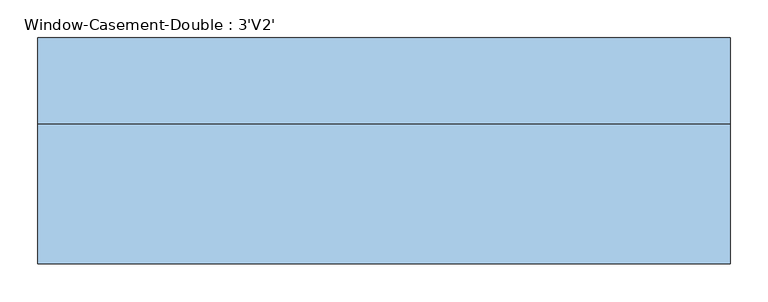
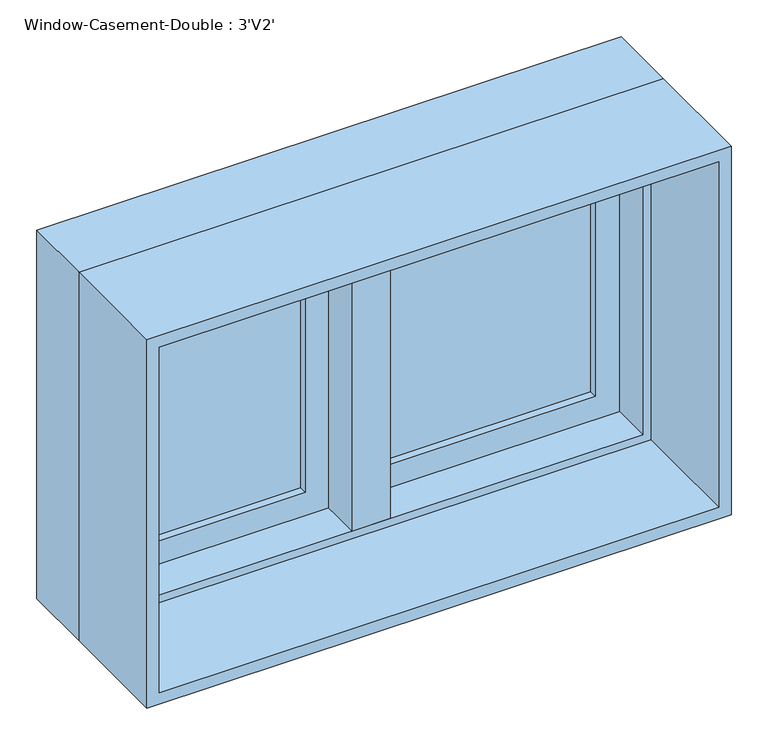
"""IFC4 building model written with IfcOpenShell, lengths in millimetres: window geometry, Window-Casement-Double : 3'V2'."""

from ifc_helpers import new_model, si_unit, frame, origin, place, context, project, spatial, polyline, outline, extrude, faceted_brep, source, transform, mapped, element, save


def window_casement_double_3_v2_9f1923e6(model_context):
    return source(origin(), model_context, "Body", "SolidModel", [
        faceted_brep([(9.525, 158.75, 1511.3), (-9.525, 158.75, 1511.3), (-9.525, 107.95, 1511.3), (9.525, 107.95, 1511.3), (9.525, 158.75, 927.1), (9.525, 107.95, 927.1), (-9.525, 107.95, 927.1), (-9.525, 158.75, 927.1), (-9.525, 107.95, 946.15), (-9.525, 107.95, 1492.25), (-30.1625, 107.95, 946.15), (-30.1625, 107.95, 1492.25), (-30.1625, 44.45, 946.15), (-30.1625, 44.45, 1492.25), (30.1625, 44.45, 946.15), (30.1625, 44.45, 1492.25), (30.1625, 107.95, 946.15), (30.1625, 107.95, 1492.25), (9.525, 107.95, 946.15), (9.525, 107.95, 1492.25)], [[[0, 1, 2, 3]], [[4, 5, 6, 7]], [[1, 0, 4, 7]], [[2, 1, 7, 6, 8, 9]], [[9, 8, 10, 11]], [[11, 10, 12, 13]], [[13, 12, 14, 15]], [[15, 14, 16, 17]], [[17, 16, 18, 19]], [[0, 3, 19, 18, 5, 4]], [[18, 8, 6, 5]], [[9, 19, 3, 2]], [[8, 18, 16, 14, 12, 10]], [[19, 9, 11, 13, 15, 17]]]),
        extrude(outline(polyline([(-66.675, 139.7), (-66.675, 133.35), (-387.35, 133.35), (-387.35, 139.7), (-66.675, 139.7)])), frame((0.0, 0.0, 984.25), z_axis=(0.0, 0.0, 1.0), x_axis=(1.0, 0.0, 0.0)), (0.0, 0.0, 1.0), 469.9),
        extrude(outline(polyline([(-387.35, 120.65), (-387.35, 127.0), (-66.675, 127.0), (-66.675, 120.65), (-387.35, 120.65)])), frame((0.0, 0.0, 984.25), z_axis=(0.0, 0.0, 1.0), x_axis=(1.0, 0.0, 0.0)), (0.0, 0.0, 1.0), 469.9),
        extrude(outline(polyline([(387.35, 139.7), (387.35, 133.35), (66.675, 133.35), (66.675, 139.7), (387.35, 139.7)])), frame((0.0, 0.0, 984.25), z_axis=(0.0, 0.0, 1.0), x_axis=(1.0, 0.0, 0.0)), (0.0, 0.0, 1.0), 469.9),
        extrude(outline(polyline([(66.675, 120.65), (66.675, 127.0), (387.35, 127.0), (387.35, 120.65), (66.675, 120.65)])), frame((0.0, 0.0, 984.25), z_axis=(0.0, 0.0, 1.0), x_axis=(1.0, 0.0, 0.0)), (0.0, 0.0, 1.0), 469.9),
        extrude(outline(polyline([(1511.3, -444.5), (927.1, -444.5), (927.1, -9.525), (1511.3, -9.525), (1511.3, -444.5)]), holes=[polyline([(1454.15, -66.675), (984.25, -66.675), (984.25, -387.35), (1454.15, -387.35), (1454.15, -66.675)])]), frame((0.0, 107.95, 0.0), z_axis=(0.0, 1.0, 0.0), x_axis=(0.0, 0.0, 1.0)), (0.0, 0.0, 1.0), 44.45),
        extrude(outline(polyline([(927.1, 444.5), (1511.3, 444.5), (1511.3, 9.525), (927.1, 9.525), (927.1, 444.5)]), holes=[polyline([(984.25, 66.675), (1454.15, 66.675), (1454.15, 387.35), (984.25, 387.35), (984.25, 66.675)])]), frame((0.0, 107.95, 0.0), z_axis=(0.0, 1.0, 0.0), x_axis=(0.0, 0.0, 1.0)), (0.0, 0.0, 1.0), 44.45),
        extrude(outline(polyline([(1524.0, -457.2), (914.4, -457.2), (914.4, 457.2), (1524.0, 457.2), (1524.0, -457.2)]), holes=[polyline([(1504.95, 438.15), (933.45, 438.15), (933.45, -438.15), (1504.95, -438.15), (1504.95, 438.15)])]), frame((0.0, -139.7, 0.0), z_axis=(0.0, 1.0, 0.0), x_axis=(0.0, 0.0, 1.0)), (0.0, 0.0, 1.0), 184.15),
        faceted_brep([(425.45, 107.95, 1492.25), (425.45, 44.45, 1492.25), (-425.45, 44.45, 1492.25), (-425.45, 107.95, 1492.25), (444.5, 158.75, 1511.3), (444.5, 107.95, 1511.3), (-444.5, 107.95, 1511.3), (-444.5, 158.75, 1511.3), (457.2, 44.45, 1524.0), (457.2, 158.75, 1524.0), (-457.2, 158.75, 1524.0), (-457.2, 44.45, 1524.0), (-425.45, 44.45, 946.15), (-425.45, 107.95, 946.15), (-444.5, 107.95, 927.1), (-444.5, 158.75, 927.1), (-457.2, 158.75, 914.4), (-457.2, 44.45, 914.4), (425.45, 44.45, 946.15), (425.45, 107.95, 946.15), (444.5, 107.95, 927.1), (444.5, 158.75, 927.1), (457.2, 158.75, 914.4), (457.2, 44.45, 914.4)], [[[0, 1, 2, 3]], [[4, 5, 6, 7]], [[8, 9, 10, 11]], [[3, 2, 12, 13]], [[7, 6, 14, 15]], [[11, 10, 16, 17]], [[13, 12, 18, 19]], [[15, 14, 20, 21]], [[17, 16, 22, 23]], [[11, 17, 23, 8], [1, 18, 12, 2]], [[19, 18, 1, 0]], [[5, 20, 14, 6], [3, 13, 19, 0]], [[21, 20, 5, 4]], [[23, 22, 9, 8]], [[9, 22, 16, 10], [7, 15, 21, 4]]]),
    ])


if __name__ == "__main__":
    model = new_model("IFC4")
    model_context = context("Model", 3, world=origin())
    ifc_project = project(units=[si_unit("LENGTHUNIT", "METRE", prefix="MILLI")], contexts=[model_context])
    site = spatial("IfcSite", under=ifc_project)
    building = spatial("IfcBuilding", under=site)
    placement = place(None, origin())
    window_casement_double_3_v2_shape = window_casement_double_3_v2_9f1923e6(model_context)
    element("IfcWindow", 1, ObjectType="Window-Casement-Double : 3'V2'", at=placement, inside=building, context=model_context, shape_type="MappedRepresentation", body=[
        mapped(window_casement_double_3_v2_shape, transform((0.0, 0.0, 0.0), x_axis=(1.0, 0.0, 0.0), y_axis=(0.0, 1.0, 0.0), z_axis=(0.0, 0.0, 1.0))),
    ])
    save(model, "model.ifc")

# Revit data of these elements
# Type "Window-Casement-Double : 3'V2'"
#   Type Mark = "18"
#   Fire Rating = "0.5h"
#   Assembly Code = "B2020100"
#   Analytic Construction = "Double glazing - domestic"
#   Frame Extension [instance default] = 0.25"
#   Window Inset [instance default] = 0"
#   Wall Thickness [instance default] = 6"
#   Interior Wall Closure [instance default] = 2.25"
#   Half Width = 18"
#   Visual Light Transmittance = 0.81
#   Thermal Resistance (R) = 1.8146 (h·ft²·°F)/BTU
#   Solar Heat Gain Coefficient = 0.76
#   Rough Width = 36.5"
#   Rough Height = 24.5"
#   Height = 24"
#   Heat Transfer Coefficient (U) = 0.5511 BTU/(h·ft²·°F)
#   Exterior Wall Closure [instance default] = 1.25"
#   Extension Jamb [instance default] = 2.25"
#   Default Sill Height = 36"
#   Width = 36"
#   Muntin Visibility = yes
#   Interior Trim Visibility [instance default] = yes
#   Exterior Trim Visibility [instance default] = yes
#   Extension Jamb Visibility [instance default] = yes
#   Interior Trim Material = Wood - Stained
#   Muntin Pattern = Muntin Pattern_2x2 : Muntin Pattern_2x2
#   Interior Trim = Trim-Window-Interior-Flat : Picture Frame
#   Interior Frame Material = Wood - Stained
#   Glass Panel Material = Glass
#   Exterior Trim Material = Clad - White
#   Exterior Trim = Trim-Window-Exterior-Flat : with Sill
#   Exterior Frame Material = Clad - White
#   Wall Closure = (empty or 0)
# Element 1 (IfcWindow, "Window-Casement-Double : 3'V2'")
#   Wall Thickness = 11"
#   Extension Jamb = 7.25"
#   Materials on its faces: "Wood - Stained", "Glass", "Clad - White"
# Materials
#   "Wood - Stained": class "Wood", colour RGB 224 178 126, transparency 0, Cost = 0
#   "Glass": class "Glass", colour RGB 0 128 192, transparency 0.75, Description = "Soda Lime Glass", Cost = 0
#   "Clad - White": class "Wood", colour RGB 242 242 238, transparency 0, Cost = 0
